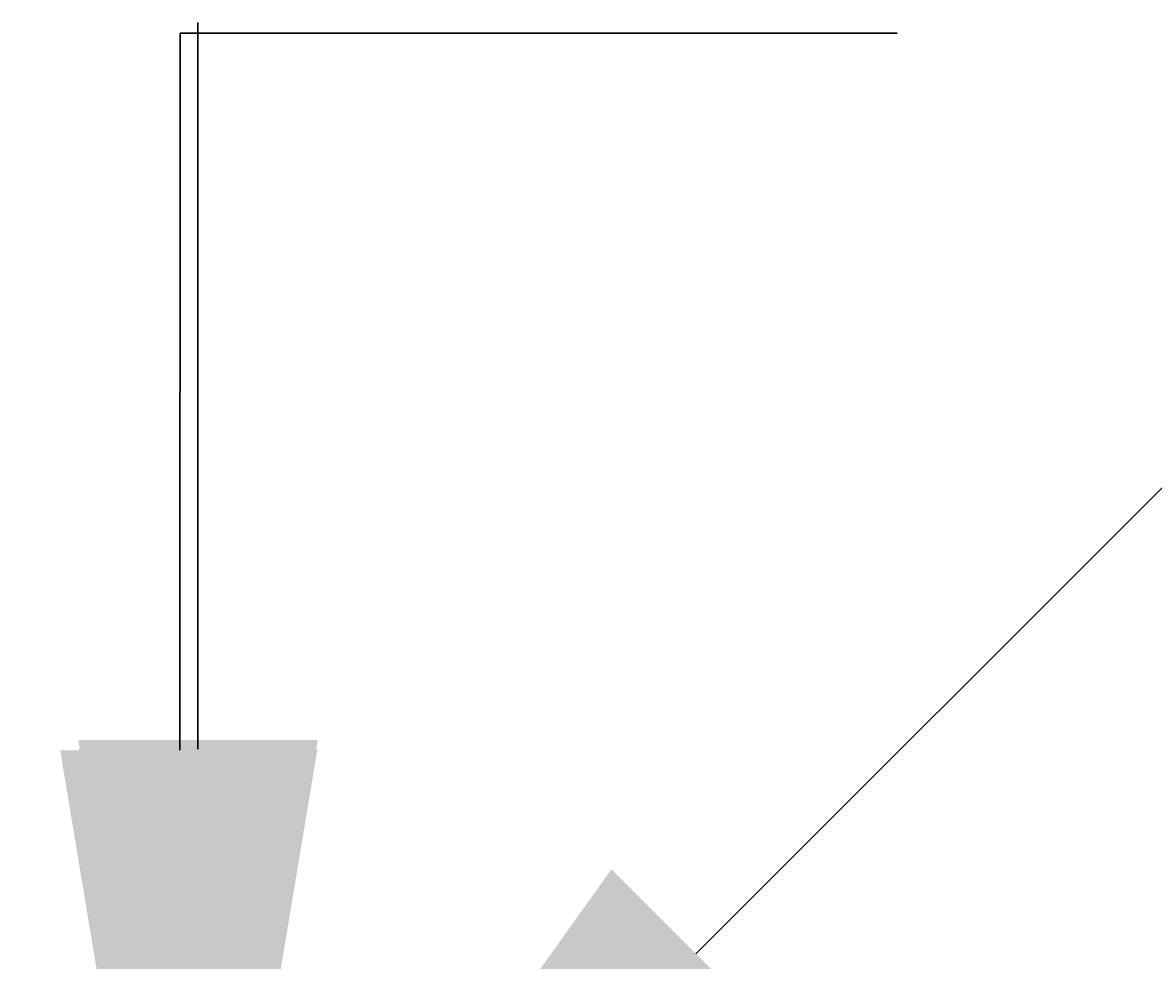
# Model space of a CAD drawing. Units: millimetres. Extents: x -22994 to 29398, y -19990 to 20176.
# Tile 134 of 135: x -2139 to 13629, y 7102 to 20176. Entities that reach past the tile are written whole.
import ezdxf

# ---------------------------------------------------------------- set-up
doc = ezdxf.new("R2010")
doc.units = ezdxf.units.MM
doc.header["$MEASUREMENT"] = 0
doc.layers.add('M-DIMS', color=2, linetype='Continuous', lineweight=18)
doc.styles.get("Standard").update_dxf_attribs({"font": 'arial.ttf'})
doc.dimstyles.get("Standard").update_dxf_attribs({"dimtxt": 0.18, "dimasz": 10000, "dimexe": 0.18, "dimexo": 0.0625, "dimgap": 0.09, "dimtad": 0, "dimtih": 1, "dimtoh": 1, "dimdec": 0, "dimzin": 0, "dimdsep": 46, "dimtxsty": 'Standard', "dimcen": 0.09, "dimadec": 0, "dimazin": 0, "dimtfac": 1, "dimtdec": 0, "dimtofl": 0, "dimtmove": 0, "dimatfit": 3, "dimfxl": 1, "dimtolj": 1, "dimtzin": 0, "dimlwd": 30, "dimarcsym": 0})

# ---------------------------------------------------------------- blocks, each defined once
blk = doc.blocks.new('*D9')
at = {"layer": 'Defpoints', "color": 0, "transparency": 16777216}
for p in [(187, 176), (306, 176), (291, 10)]:
    blk.add_point(p, dxfattribs=at)
at = {"layer": 'M-DIMS', "color": 0, "lineweight": 30, "transparency": 16777216}
for p, q in [((306, 10176), (306, 20176)), ((306, -9990), (306, -19990))]:
    blk.add_line(p, q, dxfattribs=at)
at = {"layer": 'M-DIMS', "color": 0, "lineweight": -2, "transparency": 16777216}
for p, q in [((187, 176), (306, 176)), ((291, 10), (306, 10))]:
    blk.add_line(p, q, dxfattribs=at)
at = {"layer": 'M-DIMS', "color": 0, "transparency": 16777216}
for points in [[(-1360, 10176), (1973, 10176), (306, 176)], [(-1360, -9990), (1973, -9990), (306, 10)]]:
    blk.add_solid(points, dxfattribs=at)
at = {"layer": 'M-DIMS', "color": 0, "transparency": 16777216, "insert": (306, 93), "char_height": 0.18, "attachment_point": 5}
blk.add_mtext('\\A1;166.1', dxfattribs=at)
blk = doc.blocks.new('*D15')
at = {"layer": 'Defpoints', "color": 0, "transparency": 16777216}
for p in [(173, 155), (173, 136), (306, 136)]:
    blk.add_point(p, dxfattribs=at)
at = {"layer": 'M-DIMS', "color": 0, "lineweight": 30, "transparency": 16777216}
for p, q in [((306, 10155), (306, 20155)), ((306, -9864), (306, -19864))]:
    blk.add_line(p, q, dxfattribs=at)
at = {"layer": 'M-DIMS', "color": 0, "lineweight": -2, "transparency": 16777216}
for p, q in [((173, 155), (306, 155)), ((173, 136), (306, 136))]:
    blk.add_line(p, q, dxfattribs=at)
at = {"layer": 'M-DIMS', "color": 0, "transparency": 16777216}
for points in [[(-1360, 10155), (1973, 10155), (306, 155)], [(-1360, -9864), (1973, -9864), (306, 136)]]:
    blk.add_solid(points, dxfattribs=at)
at = {"layer": 'M-DIMS', "color": 0, "transparency": 16777216, "insert": (306, 145), "char_height": 0.18, "attachment_point": 5}
blk.add_mtext('\\A1;18.717', dxfattribs=at)
blk = doc.blocks.new('*D28')
at = {"layer": 'Defpoints', "color": 0, "transparency": 16777216}
for p in [(188, 48), (188, 31), (306, 48)]:
    blk.add_point(p, dxfattribs=at)
at = {"layer": 'M-DIMS', "color": 0, "lineweight": 30, "transparency": 16777216}
for p, q in [((306, 10048), (306, 20048)), ((306, -9969), (306, -19969))]:
    blk.add_line(p, q, dxfattribs=at)
at = {"layer": 'M-DIMS', "color": 0, "lineweight": -2, "transparency": 16777216}
for p, q in [((188, 48), (306, 48)), ((188, 31), (306, 31))]:
    blk.add_line(p, q, dxfattribs=at)
at = {"layer": 'M-DIMS', "color": 0, "transparency": 16777216}
for points in [[(-1360, 10048), (1973, 10048), (306, 48)], [(-1360, -9969), (1973, -9969), (306, 31)]]:
    blk.add_solid(points, dxfattribs=at)
at = {"layer": 'M-DIMS', "color": 0, "transparency": 16777216, "insert": (306, 40), "char_height": 0.18, "attachment_point": 5}
blk.add_mtext('\\A1;17.045', dxfattribs=at)
blk = doc.blocks.new('*D34')
at = {"layer": 'Defpoints', "color": 0, "transparency": 16777216}
for p in [(177, 121), (179, 123)]:
    blk.add_point(p, dxfattribs=at)
at = {"layer": 'M-DIMS', "color": 0, "lineweight": 30, "transparency": 16777216}
for p, q in [((14322, 14263), (7251, 7193)), ((24322, 14263), (14322, 14263))]:
    blk.add_line(p, q, dxfattribs=at)
at = {"layer": 'M-DIMS', "color": 0, "lineweight": -2, "transparency": 16777216}
blk.add_line((177, 121), (177, 121), dxfattribs=at)
blk.add_line((177, 121), (177, 121), dxfattribs=at)
at = {"layer": 'M-DIMS', "color": 0, "transparency": 16777216}
blk.add_solid([(6072, 8372), (8429, 6014), (179, 123)], dxfattribs=at)
at = {"layer": 'M-DIMS', "color": 0, "transparency": 16777216, "insert": (24323, 14263), "char_height": 0.18, "attachment_point": 5}
blk.add_mtext('\\A1;6X R2.5', dxfattribs=at)
blk = doc.blocks.new('*D35')
at = {"layer": 'Defpoints', "color": 0, "transparency": 16777216}
for p in [(21, 77), (22, 76)]:
    blk.add_point(p, dxfattribs=at)
at = {"layer": 'M-DIMS', "color": 0, "lineweight": 30, "transparency": 16777216}
for p, q in [((-19938, 17421), (-9938, 17421)), ((-9938, 17421), (-4958, 8749))]:
    blk.add_line(p, q, dxfattribs=at)
at = {"layer": 'M-DIMS', "color": 0, "lineweight": -2, "transparency": 16777216}
blk.add_line((22, 76), (22, 76), dxfattribs=at)
blk.add_line((22, 76), (22, 76), dxfattribs=at)
at = {"layer": 'M-DIMS', "color": 0, "transparency": 16777216}
blk.add_solid([(-3513, 9579), (-6404, 7919), (21, 77)], dxfattribs=at)
at = {"layer": 'M-DIMS', "color": 0, "transparency": 16777216, "insert": (-19938, 17421), "char_height": 0.18, "attachment_point": 5}
blk.add_mtext('\\A1;R1.5', dxfattribs=at)
blk = doc.blocks.new('*D36')
at = {"layer": 'Defpoints', "color": 0, "transparency": 16777216}
for p in [(46, 31), (46, 27)]:
    blk.add_point(p, dxfattribs=at)
at = {"layer": 'M-DIMS', "color": 0, "lineweight": 30, "transparency": 16777216}
for p, q in [((57, 20031), (52, 10031)), ((10057, 20031), (57, 20031))]:
    blk.add_line(p, q, dxfattribs=at)
at = {"layer": 'M-DIMS', "color": 0, "lineweight": -2, "transparency": 16777216}
blk.add_line((46, 29), (46, 29), dxfattribs=at)
blk.add_line((46, 29), (46, 29), dxfattribs=at)
at = {"layer": 'M-DIMS', "color": 0, "transparency": 16777216}
blk.add_solid([(-1615, 10032), (1718, 10030), (46, 31)], dxfattribs=at)
at = {"layer": 'M-DIMS', "color": 0, "transparency": 16777216, "insert": (10058, 20031), "char_height": 0.18, "attachment_point": 5}
blk.add_mtext('\\A1;∅4.71', dxfattribs=at)

msp = doc.modelspace()

# ---------------------------------------------------------------- dimensions: what is measured, and where the dimension line sits
at = {"layer": 'M-DIMS'}
dim = msp.add_diameter_dim_2p(p1=(46.3875, 26.5934), p2=(46.39, 31.3035), dimstyle='Standard', override={"dimdec": 2, "dimlfac": 1, "dimrnd": 0, "dimzin": 0, "dimdsep": 46, "dimlunit": 2}, dxfattribs=at)
dim.commit()
dim.dimension.update_dxf_attribs({"geometry": '*D36', "text_midpoint": (10057.5542, 20031.3006), "dimtype": 163})
for base, p1, p2, override, picture, middle in [((306.202, 176.3662), (290.852, 10.2713), (187.2647, 176.3662), {"dimdec": 1, "dimlfac": 1, "dimrnd": 0, "dimzin": 0, "dimdsep": 46, "dimlunit": 2}, '*D9', (306.202, 93.3187)), ((306.202, 136.0713), (173.3459, 154.788), (173.3459, 136.0713), {"dimdec": 3, "dimlfac": 1, "dimrnd": 0, "dimzin": 0, "dimdsep": 46, "dimlunit": 2}, '*D15', (306.202, 145.4297)), ((306.202, 48.0349), (188.1175, 30.9895), (188.1175, 48.0349), {"dimdec": 3, "dimlfac": 1, "dimrnd": 0, "dimzin": 0, "dimdsep": 46, "dimlunit": 2}, '*D28', (306.202, 39.5122))]:
    dim = msp.add_linear_dim(base=base, p1=p1, p2=p2, angle=90, dimstyle='Standard', override=override, dxfattribs=at)
    dim.commit()
    dim.dimension.update_dxf_attribs({"geometry": picture, "text_midpoint": middle})
dim = msp.add_radius_dim(center=(21.8402, 76.0922), mpoint=(21.0933, 77.393), dimstyle='Standard', override={"dimdec": 1, "dimlfac": 1, "dimrnd": 0, "dimzin": 0, "dimdsep": 46, "dimlunit": 2}, dxfattribs=at)
dim.commit()
dim.dimension.update_dxf_attribs({"geometry": '*D35', "text_midpoint": (-19938.3541, 17421.4466)})
dim = msp.add_radius_dim(center=(176.8123, 121.1277), mpoint=(178.5802, 122.8952), text='6X <>', dimstyle='Standard', override={"dimdec": 1, "dimlfac": 1, "dimrnd": 0, "dimzin": 0, "dimdsep": 46, "dimlunit": 2}, dxfattribs=at)
dim.commit()
dim.dimension.update_dxf_attribs({"geometry": '*D34', "text_midpoint": (24322.9703, 14263.3108)})

doc.saveas('drawing.dxf')
